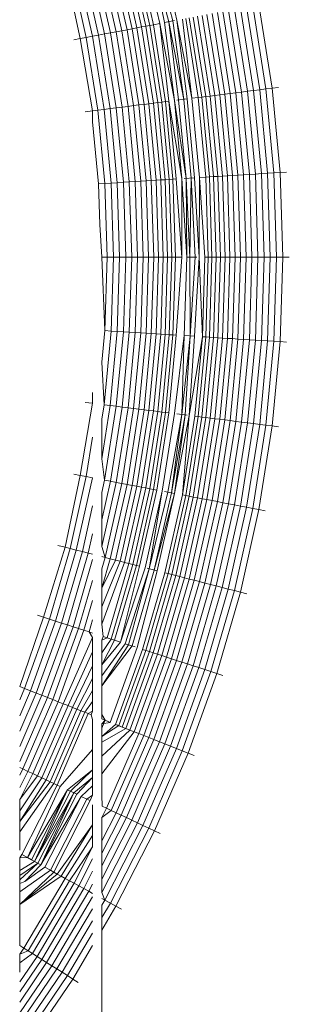
# Model space of a CAD drawing. Units: inches. Extents: x 64 to 1167, y 117 to 939.
# Tile 49 of 56: x 1130.6487 to 1130.7464, y 500.6716 to 501.0288. Entities that reach past the tile are written whole.
import ezdxf

# ---------------------------------------------------------------- set-up
doc = ezdxf.new("R2010")
doc.units = ezdxf.units.IN
doc.header["$MEASUREMENT"] = 0
doc.layers.add('A-FLOR-FIXT', color=8, linetype='Continuous', lineweight=18)

msp = doc.modelspace()

# ---------------------------------------------------------------- linework, layer by layer
at = {"layer": 'A-FLOR-FIXT'}
for p, q in [((1130.70562, 501.02864), (1130.69934, 501.05676)), ((1130.69117, 501.02588), (1130.68509, 501.0531)), ((1130.69283, 501.0262), (1130.68672, 501.05352)), ((1130.69438, 501.0265), (1130.68825, 501.05391)), ((1130.69582, 501.02677), (1130.68967, 501.05427)), ((1130.69714, 501.02702), (1130.69098, 501.05461)), ((1130.69941, 501.02745), (1130.69321, 501.05518)), ((1130.70114, 501.02779), (1130.69557, 501.05579)), ((1130.70269, 501.02808), (1130.69557, 501.05579)), ((1130.70417, 501.02836), (1130.69703, 501.05616)), ((1130.67729, 501.02323), (1130.6714, 501.04958)), ((1130.67946, 501.02365), (1130.67354, 501.05013)), ((1130.68158, 501.02405), (1130.67563, 501.05067)), ((1130.68365, 501.02445), (1130.67767, 501.05119)), ((1130.68565, 501.02483), (1130.67964, 501.0517)), ((1130.68758, 501.0252), (1130.68154, 501.05219)), ((1130.68942, 501.02555), (1130.68336, 501.05265)), ((1130.67058, 501.02196), (1130.66515, 501.04798)), ((1130.67284, 501.02239), (1130.66701, 501.04846)), ((1130.67508, 501.02281), (1130.66922, 501.04902)), ((1130.72699, 501.00232), (1130.72232, 501.03182)), ((1130.72908, 501.00258), (1130.72438, 501.03222)), ((1130.73122, 501.00285), (1130.72651, 501.03262)), ((1130.73342, 501.00313), (1130.72868, 501.03304)), ((1130.73565, 501.00341), (1130.73089, 501.03346)), ((1130.73791, 501.00369), (1130.73313, 501.03389)), ((1130.74019, 501.00398), (1130.73538, 501.03432)), ((1130.70482, 501.02849), (1130.70114, 501.02779)), ((1130.70814, 500.99993), (1130.70269, 501.02808)), ((1130.70627, 500.9997), (1130.70269, 501.02808)), ((1130.70814, 500.99993), (1130.70417, 501.02836)), ((1130.70932, 501.00008), (1130.70562, 501.02864)), ((1130.71108, 501.0003), (1130.70562, 501.02864)), ((1130.71108, 501.0003), (1130.70763, 501.02902)), ((1130.71337, 501.00059), (1130.70883, 501.02925)), ((1130.7147, 501.00076), (1130.71015, 501.0295)), ((1130.71615, 501.00095), (1130.71159, 501.02978)), ((1130.71772, 501.00114), (1130.71314, 501.03007)), ((1130.71939, 501.00135), (1130.71479, 501.03039)), ((1130.72116, 501.00158), (1130.71655, 501.03072)), ((1130.72303, 501.00181), (1130.71839, 501.03108)), ((1130.72497, 501.00206), (1130.72032, 501.03144)), ((1130.68365, 501.02445), (1130.68158, 501.02405)), ((1130.68565, 501.02483), (1130.68365, 501.02445)), ((1130.68794, 500.99738), (1130.68365, 501.02445)), ((1130.68758, 501.0252), (1130.68565, 501.02483)), ((1130.68996, 500.99764), (1130.68565, 501.02483)), ((1130.68942, 501.02555), (1130.68758, 501.0252)), ((1130.6919, 500.99788), (1130.68758, 501.0252)), ((1130.69117, 501.02588), (1130.68942, 501.02555)), ((1130.69377, 500.99812), (1130.68942, 501.02555)), ((1130.69117, 501.02588), (1130.69283, 501.0262)), ((1130.69554, 500.99834), (1130.69117, 501.02588)), ((1130.69283, 501.0262), (1130.69438, 501.0265)), ((1130.69721, 500.99855), (1130.69283, 501.0262)), ((1130.69438, 501.0265), (1130.69582, 501.02677)), ((1130.69878, 500.99875), (1130.69438, 501.0265)), ((1130.69582, 501.02677), (1130.69714, 501.02702)), ((1130.70023, 500.99893), (1130.69582, 501.02677)), ((1130.69714, 501.02702), (1130.69941, 501.02745)), ((1130.70156, 500.9991), (1130.69714, 501.02702)), ((1130.70277, 500.99926), (1130.69941, 501.02745)), ((1130.7048, 500.99951), (1130.69941, 501.02745)), ((1130.7048, 500.99951), (1130.70114, 501.02779)), ((1130.67058, 501.02196), (1130.66832, 501.02152)), ((1130.67284, 501.02239), (1130.67058, 501.02196)), ((1130.67511, 500.99576), (1130.67058, 501.02196)), ((1130.67508, 501.02281), (1130.67284, 501.02239)), ((1130.67702, 500.996), (1130.67284, 501.02239)), ((1130.67729, 501.02323), (1130.67508, 501.02281)), ((1130.67928, 500.99629), (1130.67508, 501.02281)), ((1130.67946, 501.02365), (1130.67729, 501.02323)), ((1130.68151, 500.99657), (1130.67729, 501.02323)), ((1130.68158, 501.02405), (1130.67946, 501.02365)), ((1130.68371, 500.99685), (1130.67946, 501.02365)), ((1130.68585, 500.99712), (1130.68158, 501.02405)), ((1130.73122, 501.00285), (1130.73342, 501.00313)), ((1130.73342, 501.00313), (1130.73565, 501.00341)), ((1130.73627, 500.97298), (1130.73342, 501.00313)), ((1130.73565, 501.00341), (1130.73791, 501.00369)), ((1130.73851, 500.97312), (1130.73565, 501.00341)), ((1130.73791, 501.00369), (1130.74019, 501.00398)), ((1130.74078, 500.97326), (1130.73791, 501.00369)), ((1130.74019, 501.00398), (1130.74248, 501.00427)), ((1130.74308, 500.97341), (1130.74019, 501.00398)), ((1130.70748, 500.97117), (1130.7048, 500.99951)), ((1130.70896, 500.97126), (1130.7048, 500.99951)), ((1130.70932, 501.00008), (1130.70561, 500.99961)), ((1130.70896, 500.97126), (1130.70627, 500.9997)), ((1130.71084, 500.97138), (1130.70814, 500.99993)), ((1130.71203, 500.97145), (1130.70932, 501.00008)), ((1130.71108, 501.0003), (1130.71337, 501.00059)), ((1130.71379, 500.97156), (1130.71108, 501.0003)), ((1130.71337, 501.00059), (1130.7147, 501.00076)), ((1130.7161, 500.97171), (1130.71337, 501.00059)), ((1130.7147, 501.00076), (1130.71615, 501.00095)), ((1130.71744, 500.97179), (1130.7147, 501.00076)), ((1130.71615, 501.00095), (1130.71772, 501.00114)), ((1130.7189, 500.97188), (1130.71615, 501.00095)), ((1130.71772, 501.00114), (1130.71939, 501.00135)), ((1130.72048, 500.97198), (1130.71772, 501.00114)), ((1130.71939, 501.00135), (1130.72116, 501.00158)), ((1130.72216, 500.97209), (1130.71939, 501.00135)), ((1130.72116, 501.00158), (1130.72303, 501.00181)), ((1130.72394, 500.9722), (1130.72116, 501.00158)), ((1130.72303, 501.00181), (1130.72497, 501.00206)), ((1130.72581, 500.97232), (1130.72303, 501.00181)), ((1130.72497, 501.00206), (1130.72699, 501.00232)), ((1130.72777, 500.97244), (1130.72497, 501.00206)), ((1130.72699, 501.00232), (1130.72908, 501.00258)), ((1130.7298, 500.97257), (1130.72699, 501.00232)), ((1130.72908, 501.00258), (1130.73122, 501.00285)), ((1130.7319, 500.9727), (1130.72908, 501.00258)), ((1130.73406, 500.97284), (1130.73122, 501.00285)), ((1130.67702, 500.996), (1130.67511, 500.99576)), ((1130.67928, 500.99629), (1130.67702, 500.996)), ((1130.67953, 500.96941), (1130.67702, 500.996)), ((1130.68151, 500.99657), (1130.67928, 500.99629)), ((1130.68181, 500.96955), (1130.67928, 500.99629)), ((1130.68371, 500.99685), (1130.68151, 500.99657)), ((1130.68405, 500.96969), (1130.68151, 500.99657)), ((1130.68585, 500.99712), (1130.68371, 500.99685)), ((1130.68626, 500.96983), (1130.68371, 500.99685)), ((1130.68794, 500.99738), (1130.68585, 500.99712)), ((1130.68842, 500.96997), (1130.68585, 500.99712)), ((1130.68996, 500.99764), (1130.68794, 500.99738)), ((1130.69052, 500.9701), (1130.68794, 500.99738)), ((1130.6919, 500.99788), (1130.68996, 500.99764)), ((1130.69255, 500.97023), (1130.68996, 500.99764)), ((1130.69377, 500.99812), (1130.6919, 500.99788)), ((1130.69451, 500.97035), (1130.6919, 500.99788)), ((1130.69554, 500.99834), (1130.69377, 500.99812)), ((1130.69638, 500.97047), (1130.69377, 500.99812)), ((1130.69721, 500.99855), (1130.69554, 500.99834)), ((1130.69816, 500.97058), (1130.69554, 500.99834)), ((1130.69878, 500.99875), (1130.69721, 500.99855)), ((1130.69984, 500.97069), (1130.69721, 500.99855)), ((1130.70023, 500.99893), (1130.69878, 500.99875)), ((1130.70142, 500.97078), (1130.69878, 500.99875)), ((1130.70156, 500.9991), (1130.70023, 500.99893)), ((1130.70288, 500.97088), (1130.70023, 500.99893)), ((1130.70277, 500.99926), (1130.70156, 500.9991)), ((1130.70422, 500.97096), (1130.70156, 500.9991)), ((1130.70544, 500.97104), (1130.70277, 500.99926)), ((1130.70748, 500.97117), (1130.70277, 500.99926)), ((1130.67511, 500.99576), (1130.67245, 500.99542)), ((1130.67511, 500.9918), (1130.67511, 500.99576)), ((1130.67724, 500.96926), (1130.67511, 500.9918)), ((1130.69984, 500.97069), (1130.70142, 500.97078)), ((1130.70142, 500.97078), (1130.70288, 500.97088)), ((1130.7023, 500.94271), (1130.70142, 500.97078)), ((1130.70288, 500.97088), (1130.70422, 500.97096)), ((1130.70377, 500.94271), (1130.70288, 500.97088)), ((1130.70422, 500.97096), (1130.70544, 500.97104)), ((1130.70511, 500.94271), (1130.70422, 500.97096)), ((1130.70742, 500.94271), (1130.70544, 500.97104)), ((1130.70742, 500.94271), (1130.70748, 500.97117)), ((1130.70919, 500.94271), (1130.70748, 500.97117)), ((1130.71203, 500.97145), (1130.70829, 500.97122)), ((1130.70919, 500.94271), (1130.70896, 500.97126)), ((1130.71038, 500.94271), (1130.70896, 500.97126)), ((1130.71038, 500.94271), (1130.71084, 500.97138)), ((1130.71226, 500.94271), (1130.71084, 500.97138)), ((1130.71375, 500.94271), (1130.71203, 500.97145)), ((1130.71375, 500.94271), (1130.71379, 500.97156)), ((1130.71379, 500.97156), (1130.7161, 500.97171)), ((1130.71579, 500.94271), (1130.71379, 500.97156)), ((1130.7161, 500.97171), (1130.71744, 500.97179)), ((1130.71701, 500.94271), (1130.7161, 500.97171)), ((1130.71744, 500.97179), (1130.7189, 500.97188)), ((1130.71835, 500.94271), (1130.71744, 500.97179)), ((1130.7189, 500.97188), (1130.72048, 500.97198)), ((1130.71982, 500.94271), (1130.7189, 500.97188)), ((1130.72048, 500.97198), (1130.72216, 500.97209)), ((1130.7214, 500.94271), (1130.72048, 500.97198)), ((1130.72216, 500.97209), (1130.72394, 500.9722)), ((1130.72308, 500.94271), (1130.72216, 500.97209)), ((1130.72394, 500.9722), (1130.72581, 500.97232)), ((1130.72487, 500.94271), (1130.72394, 500.9722)), ((1130.72581, 500.97232), (1130.72777, 500.97244)), ((1130.72674, 500.94271), (1130.72581, 500.97232)), ((1130.72777, 500.97244), (1130.7298, 500.97257)), ((1130.72871, 500.94271), (1130.72777, 500.97244)), ((1130.7298, 500.97257), (1130.7319, 500.9727)), ((1130.73074, 500.94271), (1130.7298, 500.97257)), ((1130.7319, 500.9727), (1130.73406, 500.97284)), ((1130.73285, 500.94271), (1130.7319, 500.9727)), ((1130.73406, 500.97284), (1130.73627, 500.97298)), ((1130.73501, 500.94271), (1130.73406, 500.97284)), ((1130.73627, 500.97298), (1130.73851, 500.97312)), ((1130.73722, 500.94271), (1130.73627, 500.97298)), ((1130.73851, 500.97312), (1130.74078, 500.97326)), ((1130.73947, 500.94271), (1130.73851, 500.97312)), ((1130.74078, 500.97326), (1130.74308, 500.97341)), ((1130.74174, 500.94271), (1130.74078, 500.97326)), ((1130.74308, 500.97341), (1130.74538, 500.97355)), ((1130.74404, 500.94271), (1130.74308, 500.97341)), ((1130.67724, 500.96926), (1130.67953, 500.96941)), ((1130.6777, 500.95456), (1130.67724, 500.96926)), ((1130.67953, 500.96941), (1130.68181, 500.96955)), ((1130.68037, 500.94271), (1130.67953, 500.96941)), ((1130.68181, 500.96955), (1130.68405, 500.96969)), ((1130.68265, 500.94271), (1130.68181, 500.96955)), ((1130.68405, 500.96969), (1130.68626, 500.96983)), ((1130.6849, 500.94271), (1130.68405, 500.96969)), ((1130.68626, 500.96983), (1130.68842, 500.96997)), ((1130.68711, 500.94271), (1130.68626, 500.96983)), ((1130.68842, 500.96997), (1130.69052, 500.9701)), ((1130.68927, 500.94271), (1130.68842, 500.96997)), ((1130.69052, 500.9701), (1130.69255, 500.97023)), ((1130.69138, 500.94271), (1130.69052, 500.9701)), ((1130.69255, 500.97023), (1130.69451, 500.97035)), ((1130.69341, 500.94271), (1130.69255, 500.97023)), ((1130.69451, 500.97035), (1130.69638, 500.97047)), ((1130.69537, 500.94271), (1130.69451, 500.97035)), ((1130.69638, 500.97047), (1130.69816, 500.97058)), ((1130.69725, 500.94271), (1130.69638, 500.97047)), ((1130.69816, 500.97058), (1130.69984, 500.97069)), ((1130.69904, 500.94271), (1130.69816, 500.97058)), ((1130.70072, 500.94271), (1130.69984, 500.97069)), ((1130.67845, 500.94271), (1130.6777, 500.95456)), ((1130.67845, 500.94271), (1130.68037, 500.94271)), ((1130.67845, 500.94271), (1130.67953, 500.91601)), ((1130.67953, 500.91601), (1130.68037, 500.94271)), ((1130.68037, 500.94271), (1130.68265, 500.94271)), ((1130.68181, 500.91586), (1130.68265, 500.94271)), ((1130.68265, 500.94271), (1130.6849, 500.94271)), ((1130.68405, 500.91572), (1130.6849, 500.94271)), ((1130.6849, 500.94271), (1130.68711, 500.94271)), ((1130.68626, 500.91558), (1130.68711, 500.94271)), ((1130.68711, 500.94271), (1130.68927, 500.94271)), ((1130.68842, 500.91545), (1130.68927, 500.94271)), ((1130.68927, 500.94271), (1130.69138, 500.94271)), ((1130.69052, 500.91532), (1130.69138, 500.94271)), ((1130.69138, 500.94271), (1130.69341, 500.94271)), ((1130.69255, 500.91519), (1130.69341, 500.94271)), ((1130.69341, 500.94271), (1130.69537, 500.94271)), ((1130.69451, 500.91507), (1130.69537, 500.94271)), ((1130.69537, 500.94271), (1130.69725, 500.94271)), ((1130.69638, 500.91495), (1130.69725, 500.94271)), ((1130.69725, 500.94271), (1130.69904, 500.94271)), ((1130.69816, 500.91484), (1130.69904, 500.94271)), ((1130.69904, 500.94271), (1130.70072, 500.94271)), ((1130.69984, 500.91473), (1130.70072, 500.94271)), ((1130.70072, 500.94271), (1130.7023, 500.94271)), ((1130.70142, 500.91463), (1130.7023, 500.94271)), ((1130.7023, 500.94271), (1130.70377, 500.94271)), ((1130.70288, 500.91454), (1130.70377, 500.94271)), ((1130.70377, 500.94271), (1130.70511, 500.94271)), ((1130.70422, 500.91445), (1130.70511, 500.94271)), ((1130.70511, 500.94271), (1130.70742, 500.94271)), ((1130.70544, 500.91438), (1130.70742, 500.94271)), ((1130.70829, 500.9142), (1130.70919, 500.94271)), ((1130.71293, 500.94271), (1130.70919, 500.94271)), ((1130.71046, 500.91406), (1130.71038, 500.94271)), ((1130.71046, 500.91406), (1130.71226, 500.94271)), ((1130.71203, 500.91396), (1130.71375, 500.94271)), ((1130.71488, 500.91378), (1130.71375, 500.94271)), ((1130.71488, 500.91378), (1130.71579, 500.94271)), ((1130.71579, 500.94271), (1130.71701, 500.94271)), ((1130.7161, 500.91371), (1130.71701, 500.94271)), ((1130.71701, 500.94271), (1130.71835, 500.94271)), ((1130.71744, 500.91362), (1130.71835, 500.94271)), ((1130.71835, 500.94271), (1130.71982, 500.94271)), ((1130.7189, 500.91353), (1130.71982, 500.94271)), ((1130.71982, 500.94271), (1130.7214, 500.94271)), ((1130.72048, 500.91343), (1130.7214, 500.94271)), ((1130.7214, 500.94271), (1130.72308, 500.94271)), ((1130.72216, 500.91333), (1130.72308, 500.94271)), ((1130.72308, 500.94271), (1130.72487, 500.94271)), ((1130.72394, 500.91321), (1130.72487, 500.94271)), ((1130.72487, 500.94271), (1130.72674, 500.94271)), ((1130.72581, 500.9131), (1130.72674, 500.94271)), ((1130.72674, 500.94271), (1130.72871, 500.94271)), ((1130.72777, 500.91297), (1130.72871, 500.94271)), ((1130.72871, 500.94271), (1130.73074, 500.94271)), ((1130.7298, 500.91285), (1130.73074, 500.94271)), ((1130.73074, 500.94271), (1130.73285, 500.94271)), ((1130.7319, 500.91271), (1130.73285, 500.94271)), ((1130.73285, 500.94271), (1130.73501, 500.94271)), ((1130.73406, 500.91258), (1130.73501, 500.94271)), ((1130.73501, 500.94271), (1130.73722, 500.94271)), ((1130.73627, 500.91244), (1130.73722, 500.94271)), ((1130.73722, 500.94271), (1130.73947, 500.94271)), ((1130.73851, 500.9123), (1130.73947, 500.94271)), ((1130.73947, 500.94271), (1130.74174, 500.94271)), ((1130.74078, 500.91215), (1130.74174, 500.94271)), ((1130.74174, 500.94271), (1130.74404, 500.94271)), ((1130.74308, 500.91201), (1130.74404, 500.94271)), ((1130.74404, 500.94271), (1130.74635, 500.94271)), ((1130.67845, 500.90452), (1130.67953, 500.91601)), ((1130.67928, 500.88913), (1130.68181, 500.91586)), ((1130.67953, 500.91601), (1130.68181, 500.91586)), ((1130.68151, 500.88885), (1130.68405, 500.91572)), ((1130.68181, 500.91586), (1130.68405, 500.91572)), ((1130.68371, 500.88857), (1130.68626, 500.91558)), ((1130.68405, 500.91572), (1130.68626, 500.91558)), ((1130.68585, 500.8883), (1130.68842, 500.91545)), ((1130.68626, 500.91558), (1130.68842, 500.91545)), ((1130.68794, 500.88803), (1130.69052, 500.91532)), ((1130.68842, 500.91545), (1130.69052, 500.91532)), ((1130.68996, 500.88778), (1130.69255, 500.91519)), ((1130.69052, 500.91532), (1130.69255, 500.91519)), ((1130.6919, 500.88753), (1130.69451, 500.91507)), ((1130.69255, 500.91519), (1130.69451, 500.91507)), ((1130.69377, 500.8873), (1130.69638, 500.91495)), ((1130.69451, 500.91507), (1130.69638, 500.91495)), ((1130.69554, 500.88707), (1130.69816, 500.91484)), ((1130.69638, 500.91495), (1130.69816, 500.91484)), ((1130.69721, 500.88686), (1130.69984, 500.91473)), ((1130.69816, 500.91484), (1130.69984, 500.91473)), ((1130.69878, 500.88666), (1130.70142, 500.91463)), ((1130.69984, 500.91473), (1130.70142, 500.91463)), ((1130.70023, 500.88648), (1130.70288, 500.91454)), ((1130.70142, 500.91463), (1130.70288, 500.91454)), ((1130.70156, 500.88631), (1130.70422, 500.91445)), ((1130.70277, 500.88616), (1130.70544, 500.91438)), ((1130.70288, 500.91454), (1130.70422, 500.91445)), ((1130.70422, 500.91445), (1130.70544, 500.91438)), ((1130.7048, 500.8859), (1130.70829, 500.9142)), ((1130.70739, 500.88558), (1130.70829, 500.9142)), ((1130.70739, 500.88558), (1130.71046, 500.91406)), ((1130.71203, 500.91396), (1130.70829, 500.9142)), ((1130.70866, 500.88542), (1130.71046, 500.91406)), ((1130.71013, 500.88523), (1130.71203, 500.91396)), ((1130.71013, 500.88523), (1130.71488, 500.91378)), ((1130.71216, 500.88497), (1130.71488, 500.91378)), ((1130.71337, 500.88482), (1130.7161, 500.91371)), ((1130.7147, 500.88465), (1130.71744, 500.91362)), ((1130.7161, 500.91371), (1130.71488, 500.91378)), ((1130.71744, 500.91362), (1130.7161, 500.91371)), ((1130.7189, 500.91353), (1130.71744, 500.91362)), ((1130.71615, 500.88447), (1130.7189, 500.91353)), ((1130.71772, 500.88427), (1130.72048, 500.91343)), ((1130.72048, 500.91343), (1130.7189, 500.91353)), ((1130.71939, 500.88406), (1130.72216, 500.91333)), ((1130.72216, 500.91333), (1130.72048, 500.91343)), ((1130.72116, 500.88384), (1130.72394, 500.91321)), ((1130.72394, 500.91321), (1130.72216, 500.91333)), ((1130.72303, 500.8836), (1130.72581, 500.9131)), ((1130.72581, 500.9131), (1130.72394, 500.91321)), ((1130.72497, 500.88336), (1130.72777, 500.91297)), ((1130.72777, 500.91297), (1130.72581, 500.9131)), ((1130.72699, 500.8831), (1130.7298, 500.91285)), ((1130.7298, 500.91285), (1130.72777, 500.91297)), ((1130.72908, 500.88284), (1130.7319, 500.91271)), ((1130.7319, 500.91271), (1130.7298, 500.91285)), ((1130.73122, 500.88257), (1130.73406, 500.91258)), ((1130.73406, 500.91258), (1130.7319, 500.91271)), ((1130.73342, 500.88229), (1130.73627, 500.91244)), ((1130.73627, 500.91244), (1130.73406, 500.91258)), ((1130.73565, 500.88201), (1130.73851, 500.9123)), ((1130.73851, 500.9123), (1130.73627, 500.91244)), ((1130.73791, 500.88172), (1130.74078, 500.91215)), ((1130.74078, 500.91215), (1130.73851, 500.9123)), ((1130.74019, 500.88143), (1130.74308, 500.91201)), ((1130.74308, 500.91201), (1130.74078, 500.91215)), ((1130.74308, 500.91201), (1130.74538, 500.91186)), ((1130.67845, 500.90452), (1130.67928, 500.88913)), ((1130.67511, 500.88965), (1130.67511, 500.89362)), ((1130.67058, 500.86346), (1130.67511, 500.88965)), ((1130.67245, 500.88999), (1130.67511, 500.88965)), ((1130.67845, 500.88387), (1130.67928, 500.88913)), ((1130.67845, 500.8695), (1130.68151, 500.88885)), ((1130.67928, 500.88913), (1130.68151, 500.88885)), ((1130.68151, 500.88885), (1130.68371, 500.88857)), ((1130.67946, 500.86177), (1130.68371, 500.88857)), ((1130.68158, 500.86136), (1130.68585, 500.8883)), ((1130.68365, 500.86097), (1130.68794, 500.88803)), ((1130.68371, 500.88857), (1130.68585, 500.8883)), ((1130.68565, 500.86059), (1130.68996, 500.88778)), ((1130.68585, 500.8883), (1130.68794, 500.88803)), ((1130.68758, 500.86022), (1130.6919, 500.88753)), ((1130.68794, 500.88803), (1130.68996, 500.88778)), ((1130.68942, 500.85987), (1130.69377, 500.8873)), ((1130.68996, 500.88778), (1130.6919, 500.88753)), ((1130.69117, 500.85953), (1130.69554, 500.88707)), ((1130.6919, 500.88753), (1130.69377, 500.8873)), ((1130.69283, 500.85922), (1130.69721, 500.88686)), ((1130.69377, 500.8873), (1130.69554, 500.88707)), ((1130.69438, 500.85892), (1130.69878, 500.88666)), ((1130.69554, 500.88707), (1130.69721, 500.88686)), ((1130.69582, 500.85865), (1130.70023, 500.88648)), ((1130.69714, 500.85839), (1130.70156, 500.88631)), ((1130.69721, 500.88686), (1130.69878, 500.88666)), ((1130.69834, 500.85816), (1130.70277, 500.88616)), ((1130.69878, 500.88666), (1130.70023, 500.88648)), ((1130.70023, 500.88648), (1130.70156, 500.88631)), ((1130.70034, 500.85778), (1130.7048, 500.8859)), ((1130.70156, 500.88631), (1130.70277, 500.88616)), ((1130.70232, 500.85741), (1130.70739, 500.88558)), ((1130.70365, 500.85715), (1130.70739, 500.88558)), ((1130.70365, 500.85715), (1130.70866, 500.88542)), ((1130.70482, 500.85693), (1130.70866, 500.88542)), ((1130.70482, 500.85693), (1130.71013, 500.88523)), ((1130.70932, 500.88533), (1130.70561, 500.8858)), ((1130.70763, 500.85639), (1130.71013, 500.88523)), ((1130.67845, 500.88387), (1130.67845, 500.8695)), ((1130.70763, 500.85639), (1130.71216, 500.88497)), ((1130.70883, 500.85616), (1130.71337, 500.88482)), ((1130.71015, 500.85591), (1130.7147, 500.88465)), ((1130.71159, 500.85564), (1130.71615, 500.88447)), ((1130.71216, 500.88497), (1130.71337, 500.88482)), ((1130.71314, 500.85534), (1130.71772, 500.88427)), ((1130.71337, 500.88482), (1130.7147, 500.88465)), ((1130.7147, 500.88465), (1130.71615, 500.88447)), ((1130.71479, 500.85503), (1130.71939, 500.88406)), ((1130.71615, 500.88447), (1130.71772, 500.88427)), ((1130.71655, 500.85469), (1130.72116, 500.88384)), ((1130.71772, 500.88427), (1130.71939, 500.88406)), ((1130.71839, 500.85434), (1130.72303, 500.8836)), ((1130.71939, 500.88406), (1130.72116, 500.88384)), ((1130.72032, 500.85397), (1130.72497, 500.88336)), ((1130.72116, 500.88384), (1130.72303, 500.8836)), ((1130.72232, 500.85359), (1130.72699, 500.8831)), ((1130.72303, 500.8836), (1130.72497, 500.88336)), ((1130.72438, 500.8532), (1130.72908, 500.88284)), ((1130.72497, 500.88336), (1130.72699, 500.8831)), ((1130.72651, 500.85279), (1130.73122, 500.88257)), ((1130.72699, 500.8831), (1130.72908, 500.88284)), ((1130.72868, 500.85238), (1130.73342, 500.88229)), ((1130.72908, 500.88284), (1130.73122, 500.88257)), ((1130.73089, 500.85196), (1130.73565, 500.88201)), ((1130.73122, 500.88257), (1130.73342, 500.88229)), ((1130.73313, 500.85153), (1130.73791, 500.88172)), ((1130.73342, 500.88229), (1130.73565, 500.88201)), ((1130.73565, 500.88201), (1130.73791, 500.88172)), ((1130.73791, 500.88172), (1130.74019, 500.88143)), ((1130.73538, 500.8511), (1130.74019, 500.88143)), ((1130.74019, 500.88143), (1130.74248, 500.88114)), ((1130.67284, 500.86303), (1130.67511, 500.87735)), ((1130.67845, 500.8695), (1130.67946, 500.86177)), ((1130.66832, 500.86389), (1130.67058, 500.86346)), ((1130.66515, 500.83744), (1130.67058, 500.86346)), ((1130.66701, 500.83696), (1130.67284, 500.86303)), ((1130.66922, 500.83639), (1130.67508, 500.8626)), ((1130.67058, 500.86346), (1130.67284, 500.86303)), ((1130.67284, 500.86303), (1130.67508, 500.8626)), ((1130.67845, 500.85724), (1130.67946, 500.86177)), ((1130.67845, 500.84734), (1130.68158, 500.86136)), ((1130.67845, 500.8377), (1130.68365, 500.86097)), ((1130.67946, 500.86177), (1130.68158, 500.86136)), ((1130.67964, 500.83372), (1130.68565, 500.86059)), ((1130.68154, 500.83323), (1130.68758, 500.86022)), ((1130.68158, 500.86136), (1130.68365, 500.86097)), ((1130.68365, 500.86097), (1130.68565, 500.86059)), ((1130.68565, 500.86059), (1130.68758, 500.86022)), ((1130.68758, 500.86022), (1130.68942, 500.85987)), ((1130.67845, 500.85724), (1130.67845, 500.84734)), ((1130.68336, 500.83276), (1130.68942, 500.85987)), ((1130.68509, 500.83232), (1130.69117, 500.85953)), ((1130.68672, 500.8319), (1130.69283, 500.85922)), ((1130.68825, 500.83151), (1130.69438, 500.85892)), ((1130.68942, 500.85987), (1130.69117, 500.85953)), ((1130.68967, 500.83114), (1130.69582, 500.85865)), ((1130.69098, 500.83081), (1130.69714, 500.85839)), ((1130.69117, 500.85953), (1130.69283, 500.85922)), ((1130.69216, 500.8305), (1130.69834, 500.85816)), ((1130.69283, 500.85922), (1130.69438, 500.85892)), ((1130.69413, 500.83), (1130.70034, 500.85778)), ((1130.69438, 500.85892), (1130.69582, 500.85865)), ((1130.69557, 500.82963), (1130.70034, 500.85778)), ((1130.69557, 500.82963), (1130.70232, 500.85741)), ((1130.69582, 500.85865), (1130.69714, 500.85839)), ((1130.69714, 500.85839), (1130.69834, 500.85816)), ((1130.69739, 500.82916), (1130.70365, 500.85715)), ((1130.69739, 500.82916), (1130.70482, 500.85693)), ((1130.69855, 500.82886), (1130.70482, 500.85693)), ((1130.70482, 500.85693), (1130.70114, 500.85763)), ((1130.70132, 500.82815), (1130.70763, 500.85639)), ((1130.7025, 500.82785), (1130.70883, 500.85616)), ((1130.7038, 500.82751), (1130.71015, 500.85591)), ((1130.70522, 500.82715), (1130.71159, 500.85564)), ((1130.70675, 500.82676), (1130.71314, 500.85534)), ((1130.70883, 500.85616), (1130.70763, 500.85639)), ((1130.70838, 500.82634), (1130.71479, 500.85503)), ((1130.71015, 500.85591), (1130.70883, 500.85616)), ((1130.71011, 500.82589), (1130.71655, 500.85469)), ((1130.71159, 500.85564), (1130.71015, 500.85591)), ((1130.71314, 500.85534), (1130.71159, 500.85564)), ((1130.71193, 500.82543), (1130.71839, 500.85434)), ((1130.71479, 500.85503), (1130.71314, 500.85534)), ((1130.71383, 500.82494), (1130.72032, 500.85397)), ((1130.71655, 500.85469), (1130.71479, 500.85503)), ((1130.7158, 500.82443), (1130.72232, 500.85359)), ((1130.71839, 500.85434), (1130.71655, 500.85469)), ((1130.71784, 500.82391), (1130.72438, 500.8532)), ((1130.72032, 500.85397), (1130.71839, 500.85434)), ((1130.72232, 500.85359), (1130.72032, 500.85397)), ((1130.72438, 500.8532), (1130.72232, 500.85359)), ((1130.72651, 500.85279), (1130.72438, 500.8532)), ((1130.6714, 500.83583), (1130.67511, 500.85243)), ((1130.71993, 500.82337), (1130.72651, 500.85279)), ((1130.72207, 500.82282), (1130.72868, 500.85238)), ((1130.72425, 500.82226), (1130.73089, 500.85196)), ((1130.72646, 500.8217), (1130.73313, 500.85153)), ((1130.72868, 500.85238), (1130.72651, 500.85279)), ((1130.73089, 500.85196), (1130.72868, 500.85238)), ((1130.72868, 500.82113), (1130.73538, 500.8511)), ((1130.73313, 500.85153), (1130.73089, 500.85196)), ((1130.73538, 500.8511), (1130.73313, 500.85153)), ((1130.73765, 500.85067), (1130.73538, 500.8511)), ((1130.67845, 500.84734), (1130.67845, 500.8377)), ((1130.67354, 500.83528), (1130.67511, 500.84231)), ((1130.65738, 500.81202), (1130.66515, 500.83744)), ((1130.65956, 500.81131), (1130.66701, 500.83696)), ((1130.66173, 500.8106), (1130.66922, 500.83639)), ((1130.66515, 500.83744), (1130.66255, 500.8381)), ((1130.66387, 500.80991), (1130.6714, 500.83583)), ((1130.66701, 500.83696), (1130.66515, 500.83744)), ((1130.66597, 500.80922), (1130.67354, 500.83528)), ((1130.66922, 500.83639), (1130.66701, 500.83696)), ((1130.6714, 500.83583), (1130.66922, 500.83639)), ((1130.67354, 500.83528), (1130.6714, 500.83583)), ((1130.67511, 500.83488), (1130.67354, 500.83528)), ((1130.67845, 500.8377), (1130.67964, 500.83372)), ((1130.66803, 500.80856), (1130.67511, 500.83294)), ((1130.67964, 500.83372), (1130.67845, 500.83402)), ((1130.67845, 500.8296), (1130.67964, 500.83372)), ((1130.67845, 500.82257), (1130.68154, 500.83323)), ((1130.67845, 500.82257), (1130.68336, 500.83276)), ((1130.67845, 500.81585), (1130.68509, 500.83232)), ((1130.67845, 500.80945), (1130.68672, 500.8319)), ((1130.68154, 500.83323), (1130.67964, 500.83372)), ((1130.68042, 500.80453), (1130.68825, 500.83151)), ((1130.68336, 500.83276), (1130.68154, 500.83323)), ((1130.68509, 500.83232), (1130.68336, 500.83276)), ((1130.68672, 500.8319), (1130.68509, 500.83232)), ((1130.68825, 500.83151), (1130.68672, 500.8319)), ((1130.68967, 500.83114), (1130.68825, 500.83151)), ((1130.67845, 500.8296), (1130.67845, 500.82257)), ((1130.68181, 500.80408), (1130.68967, 500.83114)), ((1130.68309, 500.80366), (1130.69098, 500.83081)), ((1130.68528, 500.80295), (1130.69216, 500.8305)), ((1130.68528, 500.80295), (1130.69413, 500.83)), ((1130.68696, 500.8024), (1130.69557, 500.82963)), ((1130.6881, 500.80203), (1130.69557, 500.82963)), ((1130.68939, 500.80161), (1130.69739, 500.82916)), ((1130.68967, 500.83114), (1130.69098, 500.83081)), ((1130.69098, 500.83081), (1130.69216, 500.8305)), ((1130.6913, 500.80099), (1130.69855, 500.82886)), ((1130.69324, 500.80036), (1130.70132, 500.82815)), ((1130.69855, 500.82886), (1130.69492, 500.82979)), ((1130.70132, 500.82815), (1130.7025, 500.82785)), ((1130.67003, 500.80791), (1130.67511, 500.82541)), ((1130.6944, 500.79999), (1130.7025, 500.82785)), ((1130.69568, 500.79957), (1130.7038, 500.82751)), ((1130.69707, 500.79912), (1130.70522, 500.82715)), ((1130.69858, 500.79863), (1130.70675, 500.82676)), ((1130.70018, 500.79811), (1130.70838, 500.82634)), ((1130.70188, 500.79756), (1130.71011, 500.82589)), ((1130.7025, 500.82785), (1130.7038, 500.82751)), ((1130.70366, 500.79698), (1130.71193, 500.82543)), ((1130.7038, 500.82751), (1130.70522, 500.82715)), ((1130.70522, 500.82715), (1130.70675, 500.82676)), ((1130.70553, 500.79637), (1130.71383, 500.82494)), ((1130.70675, 500.82676), (1130.70838, 500.82634)), ((1130.70746, 500.79574), (1130.7158, 500.82443)), ((1130.70838, 500.82634), (1130.71011, 500.82589)), ((1130.71011, 500.82589), (1130.71193, 500.82543)), ((1130.71193, 500.82543), (1130.71383, 500.82494)), ((1130.71383, 500.82494), (1130.7158, 500.82443)), ((1130.7158, 500.82443), (1130.71784, 500.82391)), ((1130.67845, 500.81585), (1130.67845, 500.82257)), ((1130.70947, 500.79509), (1130.71784, 500.82391)), ((1130.71152, 500.79442), (1130.71993, 500.82337)), ((1130.71362, 500.79374), (1130.72207, 500.82282)), ((1130.71576, 500.79305), (1130.72425, 500.82226)), ((1130.71784, 500.82391), (1130.71993, 500.82337)), ((1130.71793, 500.79234), (1130.72646, 500.8217)), ((1130.71993, 500.82337), (1130.72207, 500.82282)), ((1130.72012, 500.79163), (1130.72868, 500.82113)), ((1130.72207, 500.82282), (1130.72425, 500.82226)), ((1130.72425, 500.82226), (1130.72646, 500.8217)), ((1130.72646, 500.8217), (1130.72868, 500.82113)), ((1130.72868, 500.82113), (1130.73092, 500.82055)), ((1130.67196, 500.80728), (1130.67511, 500.81811)), ((1130.67845, 500.80945), (1130.67845, 500.81585)), ((1130.64872, 500.78688), (1130.65738, 500.81202)), ((1130.65051, 500.78617), (1130.65956, 500.81131)), ((1130.65263, 500.78533), (1130.66173, 500.8106)), ((1130.65518, 500.81273), (1130.65738, 500.81202)), ((1130.65738, 500.81202), (1130.65956, 500.81131)), ((1130.65956, 500.81131), (1130.66173, 500.8106)), ((1130.66173, 500.8106), (1130.66387, 500.80991)), ((1130.67383, 500.80667), (1130.67511, 500.81108)), ((1130.65472, 500.78451), (1130.66387, 500.80991)), ((1130.65678, 500.78369), (1130.66597, 500.80922)), ((1130.65879, 500.7829), (1130.66803, 500.80856)), ((1130.66074, 500.78212), (1130.67003, 500.80791)), ((1130.66264, 500.78137), (1130.67196, 500.80728)), ((1130.66387, 500.80991), (1130.66597, 500.80922)), ((1130.66597, 500.80922), (1130.66803, 500.80856)), ((1130.66803, 500.80856), (1130.67003, 500.80791)), ((1130.67003, 500.80791), (1130.67196, 500.80728)), ((1130.67196, 500.80728), (1130.67383, 500.80667)), ((1130.67383, 500.80667), (1130.67511, 500.80625)), ((1130.67511, 500.80469), (1130.67383, 500.80667)), ((1130.67891, 500.80502), (1130.67845, 500.80945)), ((1130.66446, 500.78065), (1130.67511, 500.80469)), ((1130.67511, 500.79943), (1130.67511, 500.80469)), ((1130.67845, 500.80372), (1130.67891, 500.80502)), ((1130.67845, 500.80372), (1130.68042, 500.80453)), ((1130.67845, 500.79907), (1130.68181, 500.80408)), ((1130.67845, 500.79907), (1130.67845, 500.80372)), ((1130.67845, 500.79474), (1130.68309, 500.80366)), ((1130.67845, 500.79474), (1130.68528, 500.80295)), ((1130.67891, 500.80502), (1130.68042, 500.80453)), ((1130.68042, 500.80453), (1130.68181, 500.80408)), ((1130.68309, 500.80366), (1130.68181, 500.80408)), ((1130.68528, 500.80295), (1130.68309, 500.80366)), ((1130.66621, 500.77996), (1130.67511, 500.79943)), ((1130.67511, 500.79445), (1130.67511, 500.79943)), ((1130.67845, 500.79077), (1130.68696, 500.8024)), ((1130.67845, 500.78717), (1130.6881, 500.80203)), ((1130.67845, 500.78717), (1130.68939, 500.80161)), ((1130.68154, 500.77389), (1130.6913, 500.80099)), ((1130.68344, 500.77314), (1130.69324, 500.80036)), ((1130.68457, 500.77269), (1130.6944, 500.79999)), ((1130.68582, 500.77219), (1130.69568, 500.79957)), ((1130.69053, 500.80125), (1130.68696, 500.8024)), ((1130.69324, 500.80036), (1130.6944, 500.79999)), ((1130.6944, 500.79999), (1130.69568, 500.79957)), ((1130.69568, 500.79957), (1130.69707, 500.79912)), ((1130.67845, 500.79474), (1130.67845, 500.79907)), ((1130.68719, 500.77165), (1130.69707, 500.79912)), ((1130.68865, 500.77107), (1130.69858, 500.79863)), ((1130.69022, 500.77045), (1130.70018, 500.79811)), ((1130.69188, 500.76979), (1130.70188, 500.79756)), ((1130.69363, 500.7691), (1130.70366, 500.79698)), ((1130.69545, 500.76838), (1130.70553, 500.79637)), ((1130.69707, 500.79912), (1130.69858, 500.79863)), ((1130.69734, 500.76763), (1130.70746, 500.79574)), ((1130.69858, 500.79863), (1130.70018, 500.79811)), ((1130.70018, 500.79811), (1130.70188, 500.79756)), ((1130.70188, 500.79756), (1130.70366, 500.79698)), ((1130.70366, 500.79698), (1130.70553, 500.79637)), ((1130.70553, 500.79637), (1130.70746, 500.79574)), ((1130.70746, 500.79574), (1130.70947, 500.79509)), ((1130.66787, 500.7793), (1130.67511, 500.79445)), ((1130.67511, 500.78979), (1130.67511, 500.79445)), ((1130.67845, 500.79077), (1130.67845, 500.79474)), ((1130.6993, 500.76686), (1130.70947, 500.79509)), ((1130.70131, 500.76606), (1130.71152, 500.79442)), ((1130.70336, 500.76525), (1130.71362, 500.79374)), ((1130.70546, 500.76442), (1130.71576, 500.79305)), ((1130.70757, 500.76358), (1130.71793, 500.79234)), ((1130.70947, 500.79509), (1130.71152, 500.79442)), ((1130.71152, 500.79442), (1130.71362, 500.79374)), ((1130.71362, 500.79374), (1130.71576, 500.79305)), ((1130.71576, 500.79305), (1130.71793, 500.79234)), ((1130.71793, 500.79234), (1130.72012, 500.79163)), ((1130.66943, 500.77868), (1130.67511, 500.78979)), ((1130.67511, 500.78547), (1130.67511, 500.78979)), ((1130.67845, 500.78717), (1130.67845, 500.79077)), ((1130.70971, 500.76273), (1130.72012, 500.79163)), ((1130.72012, 500.79163), (1130.72231, 500.79092)), ((1130.64872, 500.78688), (1130.65051, 500.78617)), ((1130.64872, 500.78204), (1130.65051, 500.78617)), ((1130.64872, 500.7763), (1130.65263, 500.78533)), ((1130.65051, 500.78617), (1130.65263, 500.78533)), ((1130.65263, 500.78533), (1130.65472, 500.78451)), ((1130.6709, 500.7781), (1130.67511, 500.78547)), ((1130.67511, 500.7815), (1130.67511, 500.78547)), ((1130.67845, 500.77677), (1130.67845, 500.78717)), ((1130.64872, 500.77064), (1130.65472, 500.78451)), ((1130.64872, 500.76508), (1130.65678, 500.78369)), ((1130.64872, 500.75964), (1130.65879, 500.7829)), ((1130.64986, 500.75697), (1130.66074, 500.78212)), ((1130.65472, 500.78451), (1130.65678, 500.78369)), ((1130.65678, 500.78369), (1130.65879, 500.7829)), ((1130.65879, 500.7829), (1130.66074, 500.78212)), ((1130.66074, 500.78212), (1130.66264, 500.78137)), ((1130.67226, 500.77756), (1130.67511, 500.7815)), ((1130.67511, 500.7779), (1130.67511, 500.7815)), ((1130.6517, 500.7561), (1130.66264, 500.78137)), ((1130.65348, 500.75527), (1130.66446, 500.78065)), ((1130.65518, 500.75447), (1130.66621, 500.77996)), ((1130.65679, 500.75371), (1130.66787, 500.7793)), ((1130.65832, 500.75299), (1130.66943, 500.77868)), ((1130.65974, 500.75232), (1130.6709, 500.7781)), ((1130.66264, 500.78137), (1130.66446, 500.78065)), ((1130.66446, 500.78065), (1130.66621, 500.77996)), ((1130.66621, 500.77996), (1130.66787, 500.7793)), ((1130.66787, 500.7793), (1130.66943, 500.77868)), ((1130.66943, 500.77868), (1130.6709, 500.7781)), ((1130.6709, 500.7781), (1130.67226, 500.77756)), ((1130.67351, 500.77707), (1130.67511, 500.7779)), ((1130.67465, 500.77662), (1130.67511, 500.7779)), ((1130.66107, 500.7517), (1130.67226, 500.77756)), ((1130.66229, 500.75112), (1130.67351, 500.77707)), ((1130.67226, 500.77756), (1130.67351, 500.77707)), ((1130.67351, 500.77707), (1130.67465, 500.77662)), ((1130.67511, 500.77495), (1130.67465, 500.77662)), ((1130.67511, 500.77495), (1130.67511, 500.7656)), ((1130.67967, 500.77463), (1130.67845, 500.77677)), ((1130.67845, 500.77522), (1130.67845, 500.77677)), ((1130.68079, 500.77419), (1130.67845, 500.77511)), ((1130.67845, 500.77179), (1130.67967, 500.77463)), ((1130.67845, 500.77331), (1130.67967, 500.77463)), ((1130.67967, 500.77463), (1130.68154, 500.77389)), ((1130.67845, 500.77331), (1130.68154, 500.77389)), ((1130.67845, 500.77047), (1130.67845, 500.77331)), ((1130.67845, 500.77331), (1130.67845, 500.77179)), ((1130.67845, 500.76879), (1130.68344, 500.77314)), ((1130.67845, 500.76879), (1130.68457, 500.77269)), ((1130.67845, 500.77047), (1130.67845, 500.77179)), ((1130.67845, 500.76879), (1130.67845, 500.77179)), ((1130.67845, 500.76674), (1130.68719, 500.77165)), ((1130.67845, 500.7616), (1130.68865, 500.77107)), ((1130.68344, 500.77314), (1130.68457, 500.77269)), ((1130.68344, 500.77314), (1130.68582, 500.77219)), ((1130.68457, 500.77269), (1130.68582, 500.77219)), ((1130.68582, 500.77219), (1130.68719, 500.77165)), ((1130.68719, 500.77165), (1130.68865, 500.77107)), ((1130.68865, 500.77107), (1130.69022, 500.77045)), ((1130.67511, 500.7656), (1130.67511, 500.76749)), ((1130.67845, 500.76879), (1130.67845, 500.77047)), ((1130.67845, 500.75515), (1130.69022, 500.77045)), ((1130.67845, 500.76674), (1130.67845, 500.76879)), ((1130.68016, 500.74271), (1130.69188, 500.76979)), ((1130.68186, 500.74191), (1130.69363, 500.7691)), ((1130.68364, 500.74108), (1130.69545, 500.76838)), ((1130.68548, 500.74021), (1130.69734, 500.76763)), ((1130.69022, 500.77045), (1130.69188, 500.76979)), ((1130.69188, 500.76979), (1130.69363, 500.7691)), ((1130.69363, 500.7691), (1130.69545, 500.76838)), ((1130.69545, 500.76838), (1130.69734, 500.76763)), ((1130.69734, 500.76763), (1130.6993, 500.76686)), ((1130.66339, 500.7506), (1130.67511, 500.76408)), ((1130.67511, 500.76408), (1130.67511, 500.7656)), ((1130.67511, 500.75663), (1130.67511, 500.76408)), ((1130.67845, 500.76674), (1130.67845, 500.7616)), ((1130.68738, 500.73932), (1130.6993, 500.76686)), ((1130.68934, 500.73839), (1130.70131, 500.76606)), ((1130.69134, 500.73745), (1130.70336, 500.76525)), ((1130.69337, 500.7365), (1130.70546, 500.76442)), ((1130.69543, 500.73553), (1130.70757, 500.76358)), ((1130.6993, 500.76686), (1130.70131, 500.76606)), ((1130.70131, 500.76606), (1130.70336, 500.76525)), ((1130.70336, 500.76525), (1130.70546, 500.76442)), ((1130.70546, 500.76442), (1130.70757, 500.76358)), ((1130.70757, 500.76358), (1130.70971, 500.76273)), ((1130.67845, 500.75515), (1130.67845, 500.7616)), ((1130.69751, 500.73455), (1130.70971, 500.76273)), ((1130.70971, 500.76273), (1130.71186, 500.76188)), ((1130.64986, 500.75697), (1130.64872, 500.75751)), ((1130.64872, 500.75474), (1130.64986, 500.75697)), ((1130.6517, 500.7561), (1130.64986, 500.75697)), ((1130.66597, 500.74939), (1130.67511, 500.75663)), ((1130.66706, 500.74888), (1130.67511, 500.75663)), ((1130.67511, 500.75389), (1130.67511, 500.75663)), ((1130.64872, 500.75026), (1130.6517, 500.7561)), ((1130.64872, 500.74594), (1130.65348, 500.75527)), ((1130.64872, 500.74594), (1130.65518, 500.75447)), ((1130.64872, 500.74181), (1130.65679, 500.75371)), ((1130.64872, 500.73788), (1130.65832, 500.75299)), ((1130.65348, 500.75527), (1130.6517, 500.7561)), ((1130.65518, 500.75447), (1130.65348, 500.75527)), ((1130.65679, 500.75371), (1130.65518, 500.75447)), ((1130.65832, 500.75299), (1130.65679, 500.75371)), ((1130.65974, 500.75232), (1130.65832, 500.75299)), ((1130.66828, 500.7483), (1130.67511, 500.75389)), ((1130.66936, 500.74779), (1130.67511, 500.75389)), ((1130.67511, 500.75082), (1130.67511, 500.75389)), ((1130.67845, 500.75515), (1130.67845, 500.74749)), ((1130.64872, 500.73788), (1130.65974, 500.75232)), ((1130.64872, 500.73417), (1130.66107, 500.7517)), ((1130.64945, 500.72594), (1130.66229, 500.75112)), ((1130.65148, 500.72483), (1130.66339, 500.7506)), ((1130.65148, 500.72483), (1130.66597, 500.74939)), ((1130.65303, 500.72397), (1130.66597, 500.74939)), ((1130.65407, 500.7234), (1130.66597, 500.74939)), ((1130.66107, 500.7517), (1130.65974, 500.75232)), ((1130.66229, 500.75112), (1130.66107, 500.7517)), ((1130.66339, 500.7506), (1130.66229, 500.75112)), ((1130.66936, 500.74779), (1130.66597, 500.74939)), ((1130.67096, 500.74704), (1130.67511, 500.75082)), ((1130.67511, 500.74743), (1130.67511, 500.75082)), ((1130.64872, 500.74181), (1130.64872, 500.74594)), ((1130.65407, 500.7234), (1130.66706, 500.74888)), ((1130.65407, 500.7234), (1130.66828, 500.7483)), ((1130.65526, 500.72275), (1130.66828, 500.7483)), ((1130.65631, 500.72217), (1130.66828, 500.7483)), ((1130.65631, 500.72217), (1130.66936, 500.74779)), ((1130.65631, 500.72217), (1130.67096, 500.74704)), ((1130.65786, 500.72132), (1130.67096, 500.74704)), ((1130.65988, 500.72021), (1130.67305, 500.74606)), ((1130.67096, 500.74704), (1130.67305, 500.74606)), ((1130.67305, 500.74606), (1130.67511, 500.74743)), ((1130.67305, 500.74606), (1130.67427, 500.74549)), ((1130.67427, 500.74549), (1130.67511, 500.74743)), ((1130.67855, 500.74347), (1130.67845, 500.74749)), ((1130.66106, 500.71956), (1130.67427, 500.74549)), ((1130.67511, 500.73673), (1130.67511, 500.74391)), ((1130.67845, 500.73935), (1130.68016, 500.74271)), ((1130.67855, 500.74347), (1130.68016, 500.74271)), ((1130.68016, 500.74271), (1130.68186, 500.74191)), ((1130.64872, 500.73788), (1130.64872, 500.74181)), ((1130.67845, 500.73935), (1130.68186, 500.74191)), ((1130.67845, 500.7309), (1130.68364, 500.74108)), ((1130.67845, 500.72641), (1130.68548, 500.74021)), ((1130.67845, 500.73935), (1130.67845, 500.7309)), ((1130.67845, 500.72178), (1130.68738, 500.73932)), ((1130.68186, 500.74191), (1130.68364, 500.74108)), ((1130.68364, 500.74108), (1130.68548, 500.74021)), ((1130.68548, 500.74021), (1130.68738, 500.73932)), ((1130.68738, 500.73932), (1130.68934, 500.73839)), ((1130.64872, 500.73417), (1130.64872, 500.73788)), ((1130.66234, 500.71885), (1130.67511, 500.73673)), ((1130.66372, 500.71809), (1130.67511, 500.73673)), ((1130.67511, 500.7328), (1130.67511, 500.73673)), ((1130.67845, 500.71702), (1130.68934, 500.73839)), ((1130.67845, 500.71216), (1130.69134, 500.73745)), ((1130.67956, 500.70939), (1130.69337, 500.7365)), ((1130.68156, 500.70829), (1130.69543, 500.73553)), ((1130.68934, 500.73839), (1130.69134, 500.73745)), ((1130.69134, 500.73745), (1130.69337, 500.7365)), ((1130.69337, 500.7365), (1130.69543, 500.73553)), ((1130.69543, 500.73553), (1130.69751, 500.73455)), ((1130.64872, 500.72746), (1130.64872, 500.73417)), ((1130.6652, 500.71728), (1130.67511, 500.7328)), ((1130.67511, 500.72866), (1130.67511, 500.7328)), ((1130.68357, 500.70718), (1130.69751, 500.73455)), ((1130.69751, 500.73455), (1130.6996, 500.73356)), ((1130.66677, 500.71642), (1130.67511, 500.72866)), ((1130.66841, 500.71552), (1130.67511, 500.72866)), ((1130.67845, 500.7309), (1130.67845, 500.72641)), ((1130.64872, 500.7247), (1130.64945, 500.72594)), ((1130.64872, 500.7247), (1130.65148, 500.72483)), ((1130.64872, 500.72017), (1130.64872, 500.7247)), ((1130.64945, 500.72594), (1130.65148, 500.72483)), ((1130.65148, 500.72483), (1130.65303, 500.72397)), ((1130.67013, 500.71457), (1130.67511, 500.72435)), ((1130.67845, 500.72641), (1130.67845, 500.72178)), ((1130.64872, 500.72017), (1130.65407, 500.7234)), ((1130.64872, 500.7167), (1130.65526, 500.72275)), ((1130.64872, 500.7183), (1130.65526, 500.72275)), ((1130.65054, 500.71615), (1130.65631, 500.72217)), ((1130.65054, 500.71615), (1130.65786, 500.72132)), ((1130.65631, 500.72217), (1130.65303, 500.72397)), ((1130.65786, 500.72132), (1130.65988, 500.72021)), ((1130.67845, 500.72178), (1130.67845, 500.71702)), ((1130.64872, 500.71243), (1130.65988, 500.72021)), ((1130.64872, 500.7183), (1130.64872, 500.72017)), ((1130.64872, 500.70775), (1130.66106, 500.71956)), ((1130.64872, 500.70775), (1130.66234, 500.71885)), ((1130.64872, 500.71538), (1130.64872, 500.7183)), ((1130.64872, 500.7167), (1130.64872, 500.7183)), ((1130.64872, 500.70775), (1130.66372, 500.71809)), ((1130.65024, 500.69198), (1130.6652, 500.71728)), ((1130.65988, 500.72021), (1130.66106, 500.71956)), ((1130.66106, 500.71956), (1130.66234, 500.71885)), ((1130.66234, 500.71885), (1130.66372, 500.71809)), ((1130.66372, 500.71809), (1130.6652, 500.71728)), ((1130.6652, 500.71728), (1130.66677, 500.71642)), ((1130.67191, 500.71359), (1130.67511, 500.71986)), ((1130.64872, 500.71362), (1130.64872, 500.7167)), ((1130.64872, 500.71538), (1130.64872, 500.7167)), ((1130.64872, 500.71538), (1130.65054, 500.71615)), ((1130.64872, 500.71243), (1130.64872, 500.71538)), ((1130.65175, 500.69102), (1130.66677, 500.71642)), ((1130.65333, 500.69002), (1130.66841, 500.71552)), ((1130.65499, 500.68896), (1130.67013, 500.71457)), ((1130.65671, 500.68787), (1130.67191, 500.71359)), ((1130.66677, 500.71642), (1130.66841, 500.71552)), ((1130.66841, 500.71552), (1130.67013, 500.71457)), ((1130.67013, 500.71457), (1130.67191, 500.71359)), ((1130.67191, 500.71359), (1130.67376, 500.71258)), ((1130.67376, 500.71258), (1130.67511, 500.71523)), ((1130.67845, 500.71702), (1130.67845, 500.71216)), ((1130.64872, 500.71066), (1130.64872, 500.71243)), ((1130.64872, 500.70775), (1130.64872, 500.71066)), ((1130.64872, 500.70934), (1130.64872, 500.71066)), ((1130.65848, 500.68675), (1130.67376, 500.71258)), ((1130.66031, 500.68559), (1130.67511, 500.71062)), ((1130.67376, 500.71258), (1130.67511, 500.71183)), ((1130.67845, 500.71216), (1130.67956, 500.70939)), ((1130.67845, 500.71), (1130.67956, 500.70939)), ((1130.64872, 500.69583), (1130.64872, 500.70775)), ((1130.67845, 500.70751), (1130.67956, 500.70939)), ((1130.67845, 500.70303), (1130.68156, 500.70829)), ((1130.67845, 500.70751), (1130.67845, 500.70303)), ((1130.67845, 500.69852), (1130.68357, 500.70718)), ((1130.67956, 500.70939), (1130.68156, 500.70829)), ((1130.68156, 500.70829), (1130.68357, 500.70718)), ((1130.68357, 500.70718), (1130.68559, 500.70607)), ((1130.66217, 500.6844), (1130.67511, 500.70628)), ((1130.67845, 500.70303), (1130.67845, 500.69852)), ((1130.66407, 500.6832), (1130.67511, 500.70186)), ((1130.64881, 500.69288), (1130.64872, 500.69583)), ((1130.666, 500.68198), (1130.67511, 500.69739)), ((1130.67845, 500.69852), (1130.67845, 499.97088)), ((1130.64881, 500.69288), (1130.65024, 500.69198)), ((1130.66794, 500.68075), (1130.67511, 500.69288)), ((1130.64872, 500.68975), (1130.65024, 500.69198)), ((1130.64872, 500.68975), (1130.65175, 500.69102)), ((1130.64872, 500.68657), (1130.65333, 500.69002)), ((1130.64872, 500.68657), (1130.64872, 500.68975)), ((1130.64872, 500.67975), (1130.65499, 500.68896)), ((1130.65024, 500.69198), (1130.65175, 500.69102)), ((1130.65175, 500.69102), (1130.65333, 500.69002)), ((1130.65333, 500.69002), (1130.65499, 500.68896)), ((1130.65499, 500.68896), (1130.65671, 500.68787)), ((1130.64872, 500.67613), (1130.65671, 500.68787)), ((1130.64872, 500.67239), (1130.65848, 500.68675)), ((1130.64872, 500.68324), (1130.64872, 500.68657)), ((1130.64872, 500.66854), (1130.66031, 500.68559)), ((1130.65671, 500.68787), (1130.65848, 500.68675)), ((1130.65848, 500.68675), (1130.66031, 500.68559)), ((1130.66031, 500.68559), (1130.66217, 500.6844)), ((1130.64872, 500.66461), (1130.66217, 500.6844)), ((1130.64872, 500.66061), (1130.66407, 500.6832)), ((1130.64881, 500.6567), (1130.666, 500.68198)), ((1130.66217, 500.6844), (1130.66407, 500.6832)), ((1130.66407, 500.6832), (1130.666, 500.68198)), ((1130.666, 500.68198), (1130.66794, 500.68075)), ((1130.65067, 500.65534), (1130.66794, 500.68075)), ((1130.66794, 500.68075), (1130.66989, 500.67951))]:
    msp.add_line(p, q, dxfattribs=at)

doc.saveas('drawing.dxf')
